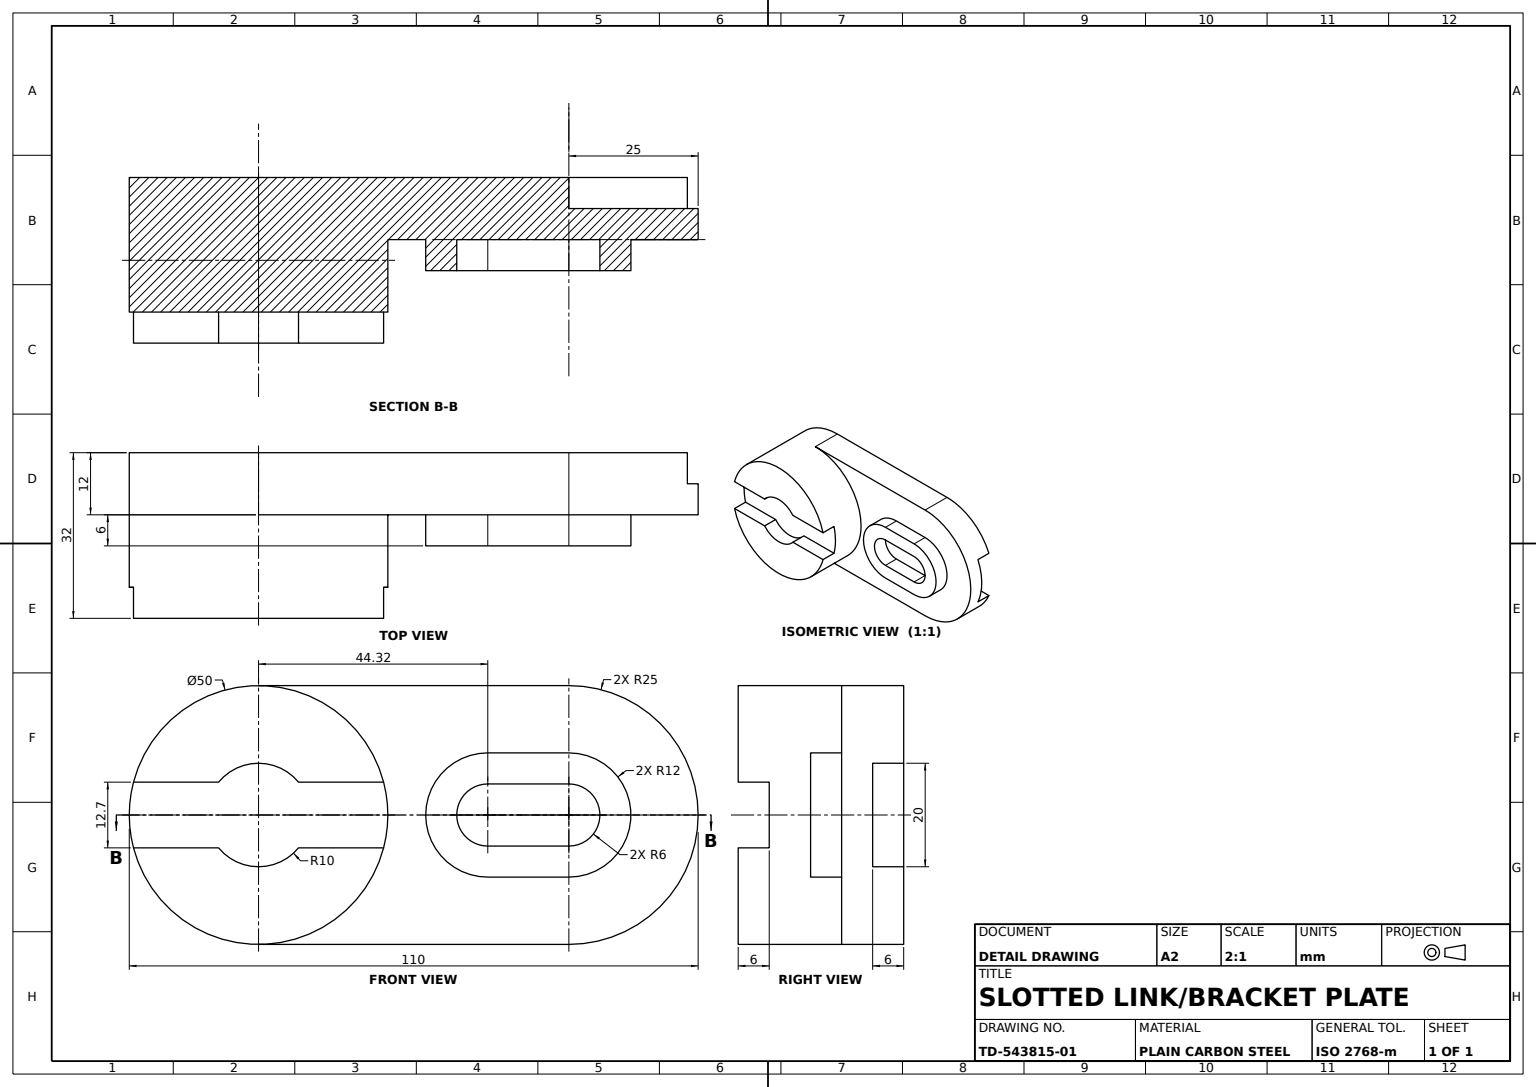
SolidWorks part; units mm, degrees
material "Plain Carbon Steel"
ref_plane "Front Plane" through (0, 0, 0) normal (0, 0, 1) x (1, 0, 0)
ref_plane "Top Plane" through (0, 0, 0) normal (0, 1, 0) x (1, 0, 0)
ref_plane "Right Plane" through (0, 0, 0) normal (1, 0, 0) x (0, 0, -1)
sketch "Base Plate Sketch" plane through (0, 0, 0) normal (0, 0, 1) x (1, 0, 0)
  line L1 (0, 25) -> (60, 25)
  line L2 (0, -25) -> (60, -25)
  arc A0 (0, 25) -> (0, -25) centre (0, 0) ccw
  arc A1 (60, -25) -> (60, 25) centre (60, 0) ccw
  dimension "D1" = 50
  dimension "D3" = 25
  dimension "D2" = 60
extrude "Base Plate" add sketch "Base Plate Sketch" along normal blind 12
sketch "Hub Boss Sketch" plane through (0, 0, 12) normal (0, 0, 1) x (1, 0, 0)
  circle A0 centre (0, 0) radius 25
  dimension "D1" = 50
extrude "Hub Boss" add sketch "Hub Boss Sketch" along normal blind 20
sketch "Hub Keyhole Slot Sketch" plane through (0, 0, 32) normal (0, 0, 1) x (1, 0, 0)
  line L0 (7.727, 6.3478) -> (24.1807, 6.3478)
  line L1 (-7.727, 6.3478) -> (-24.1807, 6.3478)
  line L3 (-7.727, -6.3478) -> (-24.1807, -6.3478)
  line L4 (7.727, -6.3478) -> (24.1807, -6.3478)
  circle A0 centre (0, 0) radius 10
  circle A1 centre (0, 0) radius 25 construction
  arc A2 (-24.1807, 6.3478) -> (-24.1807, -6.3478) centre (0, 0) ccw
  arc A3 (24.1807, -6.3478) -> (24.1807, 6.3478) centre (0, 0) ccw
  circle M6 centre (0, 0) radius 25
  dimension "D1" = 20
  dimension "D2" = 7.727
extrude "Hub Keyhole Slot" cut sketch "Hub Keyhole Slot Sketch" against normal blind 6 contours A0 L1 L3 M6 | A0 | A0 L4 L0 M6
sketch "Slot Rim Sketch" plane through (0, 0, 12) normal (0, 0, 1) x (1, 0, 0)
  line L0 (44.323, 0) -> (60, 0) construction
  line L1 (44.323, 6) -> (60, 6)
  line L2 (44.323, -6) -> (60, -6)
  line L3 (44.323, 12) -> (60, 12)
  line L4 (44.323, -12) -> (60, -12)
  arc A0 (60, -6) -> (60, 6) centre (60, 0) ccw
  arc A1 (44.323, 6) -> (44.323, -6) centre (44.323, 0) ccw
  arc A2 (44.323, 12) -> (44.323, -12) centre (44.323, 0) ccw
  arc A3 (60, -12) -> (60, 12) centre (60, 0) ccw
  point P1 (52.1615, 0)
  dimension "D1" = 12
  dimension "D2" = 6
  dimension "D3" = 44.323
extrude "Slot Rim" add sketch "Slot Rim Sketch" along normal blind 6
sketch "Obround Slot Sketch" plane through (0, 0, 0) normal (0, 0, -1) x (-1, 0, 0)
  line L1 (-82.9129, -10) -> (-60, -10)
  line L2 (-82.9129, 10) -> (-60, 10)
  line L3 (-60, 10) -> (-60, -10) construction
  arc A0 (-60, 25) -> (-60, -25) centre (-60, 0) ccw construction
  arc A1 (-82.9129, 10) -> (-82.9129, -10) centre (-60, 0) ccw
  arc M8 (-60, 25) -> (-60, -25) centre (-60, 0) ccw
  dimension "D1" = 60
  dimension "D2" = 82.9129
extrude "Obround Slot" cut sketch "Obround Slot Sketch" against normal blind 6 and the other way through all contours L3 L2 L1 M8
